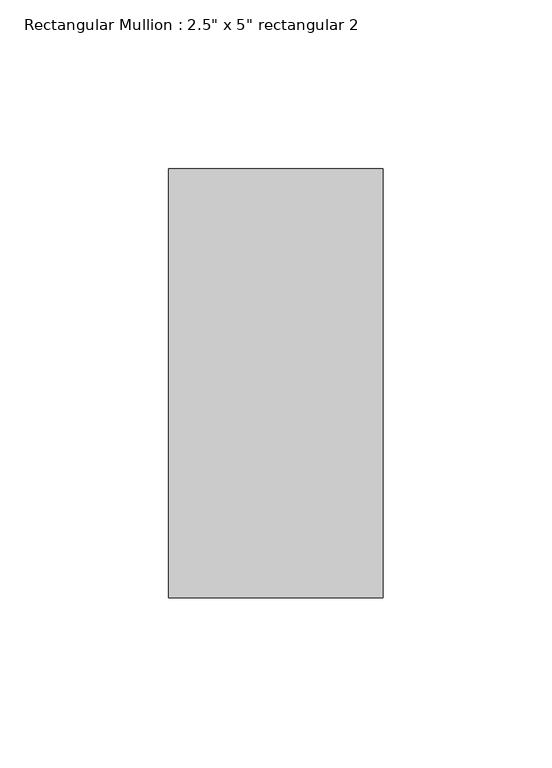
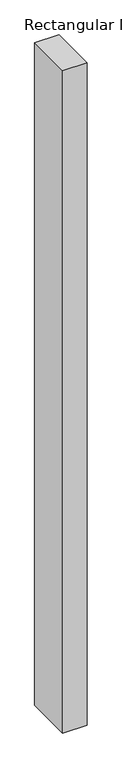
"""IFC4 building model written with IfcOpenShell, lengths in millimetres: member geometry."""

from ifc_helpers import new_model, si_unit, frame, origin, place, context, project, spatial, polyline, outline, extrude, source, transform, mapped, element, save


def member_d60e8053(model_context):
    return source(origin(), model_context, "Body", "SweptSolid", [
        extrude(outline(polyline([(31.75, 63.5), (31.75, -63.5), (-31.75, -63.5), (-31.75, 63.5), (31.75, 63.5)])), frame((0.0, 0.0, -1828.8), z_axis=(0.0, 0.0, 1.0), x_axis=(1.0, 0.0, 0.0)), (0.0, 0.0, 1.0), 1828.8),
    ])


if __name__ == "__main__":
    model = new_model("IFC4")
    model_context = context("Model", 3, world=origin())
    ifc_project = project(units=[si_unit("LENGTHUNIT", "METRE", prefix="MILLI")], contexts=[model_context])
    site = spatial("IfcSite", under=ifc_project)
    building = spatial("IfcBuilding", under=site)
    placement = place(None, origin())
    member_shape = member_d60e8053(model_context)
    element("IfcMember", 1, ObjectType="Rectangular Mullion : 2.5\" x 5\" rectangular 2", at=placement, inside=building, context=model_context, shape_type="MappedRepresentation", body=[
        mapped(member_shape, transform((0.0, 0.0, 0.0), x_axis=(1.0, 0.0, 0.0), y_axis=(0.0, 1.0, 0.0), z_axis=(0.0, 0.0, 1.0))),
    ])
    save(model, "model.ifc")

# Revit data of these elements
# Type "Rectangular Mullion : 2.5\" x 5\" rectangular 2"
#   built-in parameter 1007304 = 0.416667 (stored number, unit not read)
#   built-in parameter 1007301 = 0.104167 (stored number, unit not read)
#   built-in parameter 1007300 = 0.104167 (stored number, unit not read)
